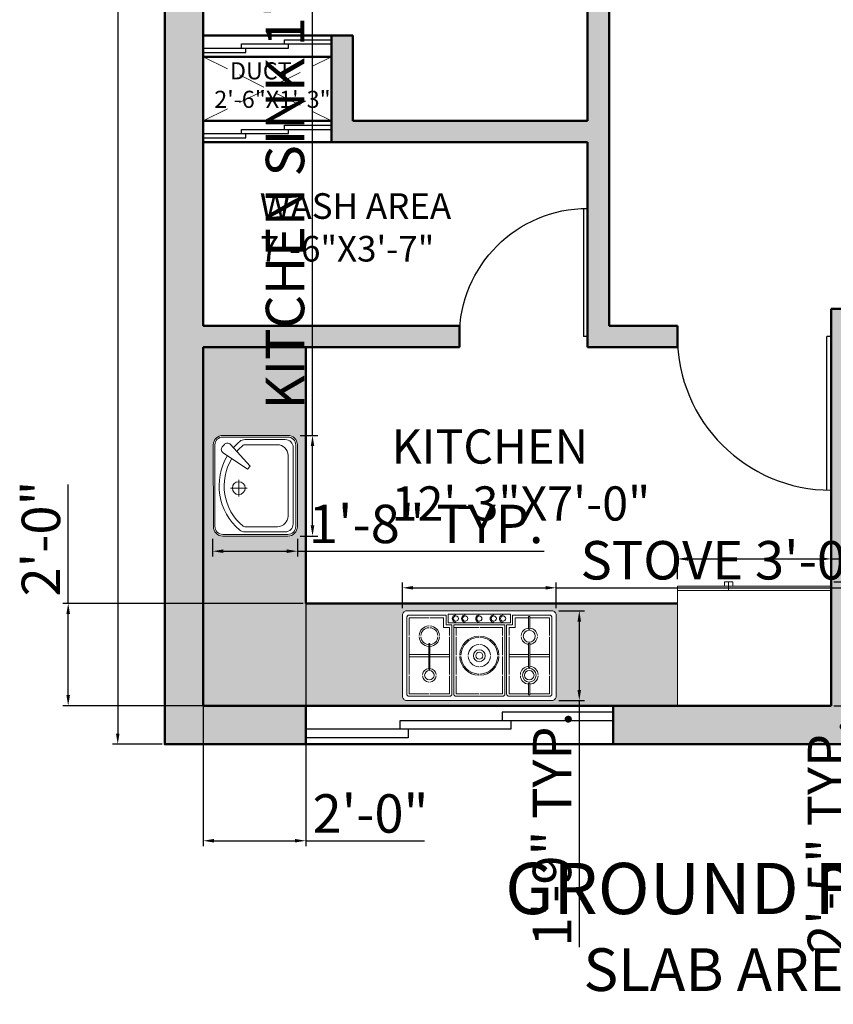
# Model space of a CAD drawing. Units: inches. Extents: x 3274 to 5176, y 1085 to 2172.
# Tile 5 of 16: x 3339 to 3530, y 1614 to 1844. Entities that reach past the tile are written whole.
import ezdxf

# ---------------------------------------------------------------- set-up
doc = ezdxf.new("R2010")
doc.units = ezdxf.units.IN
doc.linetypes.add('DASHED', pattern=[19.05, 12.7, -6.35])
for name, color, linetype, lineweight in [('A-ANNO-DIMS', 2, 'Continuous', 18), ('A-ANNO-TEXT', 7, 'Continuous', 25), ('A-AREA-IDEN', 3, 'Continuous', 25), ('A-DOOR', 4, 'Continuous', 25), ('A-FLOR-FIXT', 8, 'Continuous', 18), ('A-FLOR-OPEN', 7, 'DASHED', 18), ('A-FLOR-PATT', 252, 'Continuous', 13), ('A-GLAZ', 5, 'Continuous', 25), ('A-WALL', 7, 'Continuous', 50), ('A-WALL-PATT', 8, 'Continuous', 13)]:
    doc.layers.add(name, color=color, linetype=linetype, lineweight=lineweight)
doc.styles.get("Standard").update_dxf_attribs({"font": 'arial.ttf'})
doc.dimstyles.new('ISO-25', dxfattribs={"dimtxt": 9, "dimasz": 2.5, "dimexe": 1.25, "dimexo": 0.625, "dimtad": 1, "dimdec": 1, "dimlunit": 3, "dimtxsty": 'Standard', "dimcen": 2.5, "dimclrd": 4, "dimclre": 4, "dimclrt": 1, "dimadec": 0, "dimazin": 0, "dimtfac": 1, "dimtdec": 1, "dimtmove": 0, "dimatfit": 3, "dimfxl": 1, "dimarcsym": 0})

# ---------------------------------------------------------------- blocks, each defined once
blk = doc.blocks.new('2')
for p, q in [((0, 30), (0, 0)), ((1, 30), (1, 0)), ((0, 0), (1, 0))]:
    blk.add_line(p, q)
blk.add_arc((0, 0), 30, 0, 90)
blk = doc.blocks.new('1')
for p, q in [((0, 36), (0, 0)), ((1, 36), (1, 0)), ((0, 0), (1, 0))]:
    blk.add_line(p, q)
blk.add_arc((0, 0), 36, 0, 90)
blk = doc.blocks.new('*D68')
at = {"layer": 'A-ANNO-DIMS', "color": 0, "lineweight": -2, "transparency": 16777216}
for p, q in [((3372.68, 2034.48), (3361.05, 2034.48)), ((3362.3, 2031.98), (3362.3, 1676.98)), ((3372.68, 1674.48), (3361.05, 1674.48))]:
    blk.add_line(p, q, dxfattribs=at)
at = {"layer": 'A-ANNO-DIMS', "color": 0, "transparency": 16777216}
for points in [[(3361.88, 2031.98), (3362.71, 2031.98), (3362.3, 2034.48)], [(3361.88, 1676.98), (3362.71, 1676.98), (3362.3, 1674.48)]]:
    blk.add_solid(points, dxfattribs=at)
at = {"layer": 'Defpoints', "color": 0, "transparency": 16777216}
for p in [(3373.3, 2034.48), (3362.3, 1674.48), (3373.3, 1674.48)]:
    blk.add_point(p, dxfattribs=at)
at = {"layer": 'A-ANNO-DIMS', "color": 0, "transparency": 16777216, "insert": (3357.07, 1854.48), "char_height": 9, "attachment_point": 5, "rotation": 90}
blk.add_mtext("30'", dxfattribs=at)
blk = doc.blocks.new('STOVE')
for p, q in [((11.85, 19.7), (11.55, 19.7)), ((11.55, 16.92), (11.55, 19.7)), ((11.85, 16.92), (11.85, 19.7)), ((11.85, 16.92), (11.55, 16.92)), ((-11.85, 13.73), (-11.85, 7.62)), ((-11.85, 13.73), (-11.55, 13.73)), ((-11.55, 13.73), (-11.55, 7.62)), ((11.85, 13.23), (11.55, 13.23)), ((11.55, 13.23), (11.55, 7.57)), ((11.85, 13.23), (11.85, 7.57)), ((-11.85, 10.75), (-16.4, 10.75)), ((-11.85, 10.25), (-16.4, 10.25)), ((-7, 10.75), (-11.55, 10.75)), ((-7, 10.25), (-11.55, 10.25)), ((7, 10.75), (11.55, 10.75)), ((7, 10.25), (11.55, 10.25)), ((11.85, 10.75), (16.4, 10.75)), ((11.85, 10.25), (16.4, 10.25)), ((-11.85, 7.62), (-11.55, 7.62)), ((11.85, 7.57), (11.55, 7.57)), ((-7, 3.9), (-8.4, 3.9)), ((-7.8, 3.3), (-7.8, 1)), ((-6.4, 3.3), (-7.8, 3.3)), ((7.3, 2.8), (-7.3, 2.8)), ((-7.3, 2.8), (-7.3, 0.8)), ((-5.4, 3.9), (-6, 3.9)), ((-5.4, 3.9), (-0.15, 3.9)), ((0.15, 3.9), (5.4, 3.9)), ((6.4, 3.3), (7.8, 3.3)), ((7, 3.9), (8.4, 3.9)), ((7.3, 2.8), (7.3, 0.8)), ((7.8, 3.3), (7.8, 1)), ((8.4, 3.9), (8.4, 1.6)), ((11.85, 4.28), (11.55, 4.28)), ((11.55, 4.28), (11.55, 1.3)), ((11.85, 4.28), (11.85, 1.3)), ((7.3, 0.8), (-7.3, 0.8)), ((11.85, 1.3), (11.55, 1.3))]:
    blk.add_line(p, q)
for points in [[(-17, 21), (17, 21, -0.414214), (18, 20), (18, 1, -0.414214), (17, 0), (-17, 0, -0.414214), (-18, 1), (-18, 20, -0.414214)], [(6, 3.3), (-6, 3.3), (-6, 19.4, -0.414214), (-5.4, 20), (5.4, 20, -0.414214), (6, 19.4)]]:
    blk.add_lwpolyline(points, format="xyb", close=True)
for points in [[(-7.8, 1), (-16.4, 1, -0.414214), (-17, 1.6), (-17, 19.4, -0.414214), (-16.4, 20), (-7, 20, -0.414214), (-6.4, 19.4), (-6.4, 3.3)], [(6.4, 19.4, -0.414214), (7, 20), (16.4, 20, -0.414214), (17, 19.4), (17, 1.6, -0.414214), (16.4, 1), (7.8, 1)]]:
    blk.add_lwpolyline(points, format="xyb")
for points in [[(-16.4, 15.22), (-16.4, 19.4), (-11.85, 19.4)], [(-11.55, 19.4), (-7, 19.4), (-7, 15.22)], [(-5.4, 15.22), (-5.4, 19.4), (-0.15, 19.4)], [(0.15, 19.4), (5.4, 19.4), (5.4, 15.22)], [(6.4, 3.3), (6.4, 19.4)], [(7, 15.22), (7, 19.4), (11.55, 19.4)], [(11.85, 19.4), (16.4, 19.4), (16.4, 15.22)], [(-16.4, 6.08), (-16.4, 14.92)], [(-7, 14.92), (-7, 6.08)], [(-5.4, 10.65), (-5.4, 14.92)], [(5.4, 14.92), (5.4, 10.65)], [(7, 6.08), (7, 14.92)], [(16.4, 14.92), (16.4, 6.08)], [(-5.4, 6.08), (-5.4, 10.35)], [(5.4, 10.35), (5.4, 6.08)], [(-11.85, 1.6), (-16.4, 1.6), (-16.4, 5.77)], [(-7, 5.77), (-7, 3.9)], [(-5.4, 3.9), (-5.4, 5.77)], [(5.4, 5.77), (5.4, 3.9)], [(7, 3.9), (7, 5.77)], [(16.4, 5.77), (16.4, 1.6), (11.85, 1.6)], [(-8.4, 3.9), (-8.4, 1.6), (-11.55, 1.6)], [(11.55, 1.6), (8.4, 1.6)]]:
    blk.add_lwpolyline(points)
for centre, radius in [((-11.7, 15.07), 1.1), ((11.7, 15.07), 1.6), ((11.7, 15.07), 1.1), ((0, 10.5), 1.4), ((0, 10.5), 0.8), ((11.7, 5.93), 1.4), ((-5.49, 1.8), 0.6), ((-3.3, 1.8), 0.6), ((0, 1.8), 0.6), ((3.39, 1.8), 0.6), ((5.57, 1.8), 0.6)]:
    blk.add_circle(centre, radius)
for centre, radius, start, end in [((-11.7, 15.07), 1.6, 95.3794, 174.6206), ((-11.7, 15.07), 1.6, 5.3794, 84.6206), ((11.7, 15.07), 2.1, 94.096, 175.904), ((11.7, 15.07), 2.1, 4.096, 85.904), ((-11.7, 15.07), 1.6, 185.3794, 264.6206), ((-11.7, 15.07), 1.6, 275.3794, 354.6206), ((0, 10.5), 4.6, 91.8687, 178.1313), ((0, 10.5), 4.3, 91.9991, 178.0009), ((0, 10.5), 4.6, 1.8687, 88.1313), ((0, 10.5), 4.3, 1.9991, 88.0009), ((11.7, 15.07), 2.1, 184.096, 265.904), ((11.7, 15.07), 2.1, 274.096, 355.904), ((0, 10.5), 2.6, 93.3074, 176.6926), ((0, 10.5), 2.6, 3.3074, 86.6926), ((0, 10.5), 4.6, 181.8687, 268.1313), ((0, 10.5), 4.3, 181.9991, 268.0009), ((0, 10.5), 2.6, 183.3074, 266.6926), ((0, 10.5), 4.6, 271.8687, 358.1313), ((0, 10.5), 4.3, 271.9991, 358.0009), ((0, 10.5), 2.6, 273.3074, 356.6926), ((-11.7, 5.93), 2.4, 93.5833, 176.4167), ((-11.7, 5.93), 2, 94.3012, 175.6988), ((-11.7, 5.93), 2.4, 3.5833, 86.4167), ((-11.7, 5.93), 2, 4.3012, 85.6988), ((11.7, 5.93), 1.9, 94.5281, 175.4719), ((11.7, 5.93), 1.9, 4.5281, 85.4719), ((-11.7, 5.93), 2.4, 183.5833, 266.4167), ((-11.7, 5.93), 2, 184.3012, 265.6988), ((-11.7, 5.93), 2.4, 273.5833, 356.4167), ((-11.7, 5.93), 2, 274.3012, 355.6988), ((11.7, 5.93), 1.9, 184.5281, 265.4719), ((11.7, 5.93), 1.9, 274.5281, 355.4719), ((-5.49, 1.8), 0.846, 89.9979, 270), ((-3.3, 1.8), 0.846, 89.9979, 270), ((0, 1.8), 0.846, 89.9979, 270), ((3.39, 1.8), 0.846, 89.9979, 270), ((5.57, 1.8), 0.846, 89.9979, 270)]:
    blk.add_arc(centre, radius, start, end)
blk = doc.blocks.new('Refrigerator-2 door - 36 in top')
for p, q in [((0, -26.999999), (36, -26.999999)), ((12, -26.999999), (12, -28.999999)), ((11, -27.999999), (11, -28.999999)), ((11, -28.999999), (13, -28.999999)), ((13, -28.999999), (13, -27.999999))]:
    blk.add_line(p, q)
blk.add_lwpolyline([(0, -27.999999), (0, 0), (36, 0), (36, -27.999999)], close=True)
blk = doc.blocks.new('WIN-30')
for p, q in [((4375.19, 1317.35), (4396.19, 1317.35)), ((4375.19, 1316.35), (4375.19, 1317.35)), ((4385.19, 1318.35), (4396.19, 1318.35)), ((4385.19, 1317.35), (4385.19, 1318.35)), ((4386.19, 1316.35), (4386.19, 1317.35)), ((4366.19, 1316.35), (4386.19, 1316.35)), ((4366.19, 1315.35), (4376.19, 1315.35)), ((4376.19, 1315.35), (4376.19, 1316.35))]:
    blk.add_line(p, q)
blk = doc.blocks.new('WIN-72')
for p, q in [((4462.19, 1180.85), (4436.19, 1180.85)), ((4436.19, 1180.85), (4436.19, 1178.85)), ((4462.19, 1178.85), (4412.19, 1178.85)), ((4412.19, 1178.85), (4412.19, 1176.85)), ((4438.19, 1178.85), (4438.19, 1176.85)), ((4438.19, 1176.85), (4390.19, 1176.85)), ((4414.19, 1176.85), (4414.19, 1174.85)), ((4414.19, 1174.85), (4390.19, 1174.85))]:
    blk.add_line(p, q)
blk = doc.blocks.new('SINK-KITCHEN')
at = {"transparency": 33554687}
for points in [[(4388.24, 1243.45, 0.414214), (4386.01, 1245.69), (4370.78, 1245.67, 0.414214), (4368.55, 1243.47), (4368.57, 1224.32, 0.414214), (4370.77, 1222.1), (4386.01, 1222.1, 0.414214), (4388.24, 1224.33), (4388.24, 1243.45)], [(4387.87, 1243.45, 0.414214), (4386.01, 1245.3), (4370.78, 1245.3, 0.414214), (4368.94, 1243.47), (4368.94, 1224.32, 0.414214), (4370.77, 1222.5), (4386.01, 1222.5, 0.414214), (4387.84, 1224.33), (4387.87, 1243.45)], [(4371.89, 1240.94, 0.371519), (4374.75, 1223.51, 0.175764), (4375.92, 1223.1), (4385.42, 1223.08, 0.414214), (4387.24, 1224.93), (4387.27, 1242.85, 0.414214), (4385.41, 1244.69), (4375.92, 1244.69, 0.175764), (4374.75, 1244.27, 0.038632), (4373.27, 1242.81)], [(4372.88, 1240.28, 0.370401), (4375.51, 1224.41, 0.175764), (4375.92, 1224.28), (4383.57, 1224.28, 0.414214), (4386.06, 1226.79), (4386.06, 1241, 0.414214), (4383.55, 1243.51), (4375.92, 1243.51, 0.175764), (4375.51, 1243.36, 0.038512), (4374.06, 1241.92)]]:
    blk.add_lwpolyline(points, format="xyb", dxfattribs=at)
blk.add_lwpolyline([(4371.14, 1243.58), (4370.66, 1243, 0.463205), (4370.87, 1241.61), (4376.59, 1237.78), (4377.2, 1238.48), (4372.56, 1243.56, 0.4637)], format="xyb", close=True, dxfattribs=at)
for points in [[(4374.51, 1231.4), (4374.51, 1235.3)], [(4372.56, 1233.35), (4376.46, 1233.35)]]:
    blk.add_lwpolyline(points, dxfattribs=at)
blk.add_circle((4374.52, 1233.34), 1.5, dxfattribs=at)
blk = doc.blocks.new('*D134')
at = {"layer": 'A-ANNO-DIMS', "color": 4, "lineweight": -2, "transparency": 16777216}
for p, q in [((3428.94, 1706.35), (3428.94, 1712.37)), ((3431.44, 1711.12), (3462.44, 1711.12)), ((3464.94, 1706.35), (3464.94, 1712.37)), ((3464.94, 1711.12), (3569.61, 1711.12))]:
    blk.add_line(p, q, dxfattribs=at)
at = {"layer": 'A-ANNO-DIMS', "color": 4, "transparency": 16777216}
for points in [[(3431.44, 1711.54), (3431.44, 1710.7), (3428.94, 1711.12)], [(3462.44, 1711.54), (3462.44, 1710.7), (3464.94, 1711.12)]]:
    blk.add_solid(points, dxfattribs=at)
at = {"layer": 'Defpoints', "color": 0, "transparency": 16777216}
for p in [(3464.94, 1711.12), (3428.94, 1705.72), (3464.94, 1705.72)]:
    blk.add_point(p, dxfattribs=at)
at = {"layer": 'A-ANNO-DIMS', "color": 1, "transparency": 16777216, "insert": (3518.52, 1716.4), "char_height": 9, "attachment_point": 5}
blk.add_mtext('STOVE 3\'-0" TYP.', dxfattribs=at)
blk = doc.blocks.new('*D135')
at = {"layer": 'A-ANNO-DIMS', "color": 4, "lineweight": -2, "transparency": 16777216}
for p, q in [((3465.56, 1705.72), (3471.59, 1705.72)), ((3470.34, 1703.22), (3470.34, 1687.22)), ((3465.56, 1684.72), (3471.59, 1684.72)), ((3470.34, 1684.72), (3470.34, 1626.96))]:
    blk.add_line(p, q, dxfattribs=at)
at = {"layer": 'A-ANNO-DIMS', "color": 4, "transparency": 16777216}
for points in [[(3469.92, 1703.22), (3470.75, 1703.22), (3470.34, 1705.72)], [(3469.92, 1687.22), (3470.75, 1687.22), (3470.34, 1684.72)]]:
    blk.add_solid(points, dxfattribs=at)
at = {"layer": 'Defpoints', "color": 0, "transparency": 16777216}
for p in [(3464.94, 1705.72), (3464.94, 1684.72), (3470.34, 1684.72)]:
    blk.add_point(p, dxfattribs=at)
at = {"layer": 'A-ANNO-DIMS', "color": 1, "transparency": 16777216, "insert": (3465.12, 1654.59), "char_height": 9, "attachment_point": 5, "rotation": 90}
blk.add_mtext('1\'-9" TYP.', dxfattribs=at)
blk = doc.blocks.new('*D142')
at = {"layer": 'A-ANNO-DIMS', "color": 4, "lineweight": -2, "transparency": 16777216}
for p, q in [((3493.3, 1713.11), (3493.3, 1719.13)), ((3529.3, 1713.11), (3529.3, 1719.13)), ((3495.8, 1717.88), (3526.8, 1717.88)), ((3529.3, 1717.88), (3690.83, 1717.88))]:
    blk.add_line(p, q, dxfattribs=at)
at = {"layer": 'A-ANNO-DIMS', "color": 4, "transparency": 16777216}
for points in [[(3495.8, 1718.3), (3495.8, 1717.47), (3493.3, 1717.88)], [(3526.8, 1718.3), (3526.8, 1717.47), (3529.3, 1717.88)]]:
    blk.add_solid(points, dxfattribs=at)
at = {"layer": 'Defpoints', "color": 0, "transparency": 16777216}
for p in [(3529.3, 1717.88), (3493.3, 1712.48), (3529.3, 1712.48)]:
    blk.add_point(p, dxfattribs=at)
at = {"layer": 'A-ANNO-DIMS', "color": 1, "transparency": 16777216, "insert": (3611.31, 1723.17), "char_height": 9, "attachment_point": 5}
blk.add_mtext('REFRIGERATOR 3\'-0" TYP.', dxfattribs=at)
blk = doc.blocks.new('*D143')
at = {"layer": 'A-ANNO-DIMS', "color": 4, "lineweight": -2, "transparency": 16777216}
for p, q in [((3529.93, 1712.48), (3535.95, 1712.48)), ((3534.7, 1709.98), (3534.7, 1685.98)), ((3529.93, 1683.48), (3535.95, 1683.48)), ((3534.7, 1683.48), (3534.7, 1624.72))]:
    blk.add_line(p, q, dxfattribs=at)
at = {"layer": 'A-ANNO-DIMS', "color": 4, "transparency": 16777216}
for points in [[(3534.28, 1709.98), (3535.12, 1709.98), (3534.7, 1712.48)], [(3534.28, 1685.98), (3535.12, 1685.98), (3534.7, 1683.48)]]:
    blk.add_solid(points, dxfattribs=at)
at = {"layer": 'Defpoints', "color": 0, "transparency": 16777216}
for p in [(3529.3, 1712.48), (3529.3, 1683.48), (3534.7, 1683.48)]:
    blk.add_point(p, dxfattribs=at)
at = {"layer": 'A-ANNO-DIMS', "color": 1, "transparency": 16777216, "insert": (3529.48, 1652.85), "char_height": 9, "attachment_point": 5, "rotation": 90}
blk.add_mtext('2\'-5" TYP.', dxfattribs=at)
blk = doc.blocks.new('*D146')
at = {"layer": 'A-ANNO-DIMS', "color": 4, "lineweight": -2, "transparency": 16777216}
for p, q in [((3407.89, 1746.82), (3407.89, 1924.51)), ((3404.98, 1746.82), (3409.14, 1746.82)), ((3407.89, 1725.73), (3407.89, 1744.32)), ((3404.98, 1723.23), (3409.14, 1723.23))]:
    blk.add_line(p, q, dxfattribs=at)
at = {"layer": 'A-ANNO-DIMS', "color": 4, "transparency": 16777216}
for points in [[(3407.48, 1744.32), (3408.31, 1744.32), (3407.89, 1746.82)], [(3407.48, 1725.73), (3408.31, 1725.73), (3407.89, 1723.23)]]:
    blk.add_solid(points, dxfattribs=at)
at = {"layer": 'Defpoints', "color": 0, "transparency": 16777216}
for p in [(3404.36, 1746.82), (3407.89, 1746.82), (3404.36, 1723.23)]:
    blk.add_point(p, dxfattribs=at)
at = {"layer": 'A-ANNO-DIMS', "color": 1, "transparency": 16777216, "insert": (3402.62, 1836.92), "char_height": 9, "attachment_point": 5, "rotation": 90}
blk.add_mtext('KITCHEN SINK 1\'-11 1/2" TYP.', dxfattribs=at)
blk = doc.blocks.new('*D147')
at = {"layer": 'A-ANNO-DIMS', "color": 4, "lineweight": -2, "transparency": 16777216}
for p, q in [((3384.51, 1722.61), (3384.51, 1718.44)), ((3404.36, 1722.61), (3404.36, 1718.44)), ((3387.01, 1719.69), (3401.86, 1719.69)), ((3404.36, 1719.69), (3462.12, 1719.69))]:
    blk.add_line(p, q, dxfattribs=at)
at = {"layer": 'A-ANNO-DIMS', "color": 4, "transparency": 16777216}
for points in [[(3387.01, 1720.11), (3387.01, 1719.28), (3384.51, 1719.69)], [(3401.86, 1720.11), (3401.86, 1719.28), (3404.36, 1719.69)]]:
    blk.add_solid(points, dxfattribs=at)
at = {"layer": 'Defpoints', "color": 0, "transparency": 16777216}
for p in [(3384.51, 1723.23), (3404.36, 1723.23), (3404.36, 1719.69)]:
    blk.add_point(p, dxfattribs=at)
at = {"layer": 'A-ANNO-DIMS', "color": 1, "transparency": 16777216, "insert": (3434.49, 1724.91), "char_height": 9, "attachment_point": 5}
blk.add_mtext('1\'-8" TYP.', dxfattribs=at)
blk = doc.blocks.new('*D170')
at = {"layer": 'A-ANNO-DIMS', "color": 4, "lineweight": -2, "transparency": 16777216}
for p, q in [((3382.3, 1766.86), (3382.3, 1650.63)), ((3406.3, 1766.86), (3406.3, 1650.63)), ((3384.8, 1651.88), (3403.8, 1651.88)), ((3406.3, 1651.88), (3434.13, 1651.88))]:
    blk.add_line(p, q, dxfattribs=at)
at = {"layer": 'A-ANNO-DIMS', "color": 4, "transparency": 16777216}
for points in [[(3384.8, 1652.3), (3384.8, 1651.47), (3382.3, 1651.88)], [(3403.8, 1652.3), (3403.8, 1651.47), (3406.3, 1651.88)]]:
    blk.add_solid(points, dxfattribs=at)
at = {"layer": 'Defpoints', "color": 0, "transparency": 16777216}
for p in [(3382.3, 1767.48), (3406.3, 1767.48), (3406.3, 1651.88)]:
    blk.add_point(p, dxfattribs=at)
at = {"layer": 'A-ANNO-DIMS', "color": 1, "transparency": 16777216, "insert": (3421.46, 1657.1), "char_height": 9, "attachment_point": 5}
blk.add_mtext('2\'-0"', dxfattribs=at)
blk = doc.blocks.new('*D171')
at = {"layer": 'A-ANNO-DIMS', "color": 4, "lineweight": -2, "transparency": 16777216}
for p, q in [((3350.7, 1707.48), (3350.7, 1735.31)), ((3405.68, 1707.48), (3349.45, 1707.48)), ((3350.7, 1685.98), (3350.7, 1704.98)), ((3405.68, 1683.48), (3349.45, 1683.48))]:
    blk.add_line(p, q, dxfattribs=at)
at = {"layer": 'A-ANNO-DIMS', "color": 4, "transparency": 16777216}
for points in [[(3350.28, 1704.98), (3351.12, 1704.98), (3350.7, 1707.48)], [(3350.28, 1685.98), (3351.12, 1685.98), (3350.7, 1683.48)]]:
    blk.add_solid(points, dxfattribs=at)
at = {"layer": 'Defpoints', "color": 0, "transparency": 16777216}
for p in [(3350.7, 1707.48), (3406.3, 1707.48), (3406.3, 1683.48)]:
    blk.add_point(p, dxfattribs=at)
at = {"layer": 'A-ANNO-DIMS', "color": 1, "transparency": 16777216, "insert": (3345.48, 1722.65), "char_height": 9, "attachment_point": 5, "rotation": 90}
blk.add_mtext('2\'-0"', dxfattribs=at)

msp = doc.modelspace()

# ---------------------------------------------------------------- hatches: boundary and pattern name
at = {"layer": 'A-FLOR-PATT'}
h = msp.add_hatch(color=256, dxfattribs=at)
h.dxf.hatch_style = 1
h.paths.add_polyline_path([(3493.3, 1707.48), (3406.3, 1707.48), (3406.3, 1767.48), (3382.3, 1767.48), (3382.3, 1683.48), (3493.3, 1683.48)])
h.paths.add_polyline_path([(3404.35, 1725.46), (3404.35, 1744.59, 0.415106), (3402.11, 1746.82), (3386.86, 1746.8, 0.414031), (3384.66, 1744.55), (3384.68, 1725.43, 0.413504), (3386.9, 1723.23), (3402.13, 1723.23, 0.414214)], flags=16)
h.paths.add_polyline_path([(3386.89, 1723.63, -0.414214), (3385.05, 1725.45), (3385.05, 1744.58, -0.414214), (3386.89, 1746.43), (3402.13, 1746.43, -0.414214), (3403.98, 1744.58), (3403.96, 1725.46, -0.414214), (3402.13, 1723.63)], flags=0)
h.paths.add_polyline_path([(3392.04, 1724.23, -0.184883), (3390.82, 1724.68, -0.369938), (3388, 1742.06), (3386.98, 1742.74, -0.451108), (3386.75, 1744.1), (3387.23, 1744.68, -0.443262), (3388.6, 1744.76), (3389.37, 1743.92, -0.038991), (3390.86, 1745.39, -0.176171), (3392.04, 1745.82), (3401.52, 1745.82, -0.414214), (3403.38, 1743.98), (3403.36, 1726.06, -0.414214), (3401.53, 1724.21)], flags=0)
h.paths.add_polyline_path([(3389.14, 1734.48), (3390.62, 1734.48), (3390.62, 1735.97, 0.40968)], flags=0)
h.paths.add_polyline_path([(3428.94, 1704.72, -0.414214), (3429.94, 1705.72), (3463.94, 1705.72, -0.414214), (3464.94, 1704.72), (3464.94, 1685.72, -0.414214), (3463.94, 1684.72), (3429.94, 1684.72, -0.414214), (3428.94, 1685.72)], flags=16)
h.paths.add_polyline_path([(3429.94, 1704.12, -0.414214), (3430.54, 1704.72), (3439.14, 1704.72), (3439.14, 1702.42), (3440.54, 1702.42), (3440.54, 1686.32, -0.414214), (3439.94, 1685.72), (3430.54, 1685.72, -0.414214), (3429.94, 1686.32)], flags=0)
h.paths.add_polyline_path([(3429.94, 1699.95), (3430.54, 1699.95), (3430.54, 1704.12), (3435.09, 1704.12), (3435.09, 1704.42), (3435.39, 1704.42), (3438.54, 1704.12), (3438.54, 1701.82), (3439.94, 1701.82), (3439.94, 1699.95), (3440.54, 1699.95), (3440.54, 1699.65), (3439.94, 1699.65), (3439.94, 1690.8), (3440.54, 1690.8), (3440.54, 1690.5), (3439.94, 1690.5), (3439.94, 1686.32), (3435.39, 1686.32), (3435.39, 1686.02), (3435.09, 1686.02), (3430.54, 1686.32), (3430.54, 1690.5), (3429.94, 1690.5), (3429.94, 1690.8), (3430.54, 1690.8), (3430.54, 1699.65), (3429.94, 1699.65)], flags=0)
h.paths.add_polyline_path([(3435.39, 1702.19), (3435.39, 1701.79, -0.370891), (3437.23, 1699.95, -0.414214), (3435.39, 1697.8), (3435.39, 1697.4, 0.378035), (3437.63, 1699.65, 0.414214)], flags=0)
h.paths.add_polyline_path([(3435.09, 1689.05), (3435.09, 1689.56, -0.374693), (3434.14, 1690.65), (3433.66, 1690.36, 0.335495)], flags=0)
h.paths.add_polyline_path([(3439.64, 1702.92), (3439.64, 1704.92), (3454.24, 1704.92), (3454.24, 1702.92)], flags=0)
h.paths.add_polyline_path([(3442.05, 1703.92, -1), (3440.85, 1703.92, -1)], flags=0)
h.paths.add_polyline_path([(3440.94, 1702.42), (3452.94, 1702.42), (3452.94, 1686.32, -0.414214), (3452.34, 1685.72), (3441.54, 1685.72, -0.414214), (3440.94, 1686.32)], flags=0)
h.paths.add_polyline_path([(3440.94, 1699.95), (3441.54, 1699.95), (3441.54, 1701.82), (3446.79, 1701.82), (3446.79, 1702.12), (3447.09, 1702.12), (3452.34, 1701.82), (3452.34, 1699.95), (3452.94, 1699.95), (3452.94, 1699.65), (3452.34, 1699.65), (3452.34, 1695.37), (3452.64, 1695.37), (3452.64, 1695.07), (3452.34, 1690.8), (3452.94, 1690.8), (3452.94, 1690.5), (3452.34, 1690.5), (3452.34, 1686.32), (3447.09, 1686.32), (3447.09, 1686.02), (3446.79, 1686.02), (3441.54, 1686.32), (3441.54, 1690.5), (3440.94, 1690.5), (3440.94, 1690.8), (3441.54, 1690.8), (3441.54, 1695.07), (3441.24, 1695.07), (3441.24, 1695.37), (3441.54, 1699.65), (3440.94, 1699.65)], flags=0)
h.paths.add_polyline_path([(3447.09, 1699.82), (3447.09, 1699.52, -0.414214), (3451.23, 1695.07), (3451.53, 1695.07, 0.414214)], flags=0)
h.paths.add_polyline_path([(3444.34, 1695.37, -0.38079), (3446.79, 1697.82, -0.414214), (3449.53, 1695.37, -0.448446), (3446.79, 1692.62), (3446.79, 1690.62, -0.414214), (3442.34, 1695.37)], flags=0)
h.paths.add_polyline_path([(3444.24, 1703.92, -1), (3443.04, 1703.92, -1)], flags=0)
h.paths.add_polyline_path([(3448.34, 1695.22, -1), (3445.54, 1695.22, -1)], flags=0)
h.paths.add_polyline_path([(3447.54, 1703.92, -1), (3446.34, 1703.92, -1)], flags=0)
h.paths.add_polyline_path([(3447.74, 1695.22, -1), (3446.14, 1695.22, -1)], flags=0)
h.paths.add_polyline_path([(3450.92, 1703.92, -1), (3449.72, 1703.92, -1)], flags=0)
h.paths.add_polyline_path([(3453.11, 1703.92, -1), (3451.91, 1703.92, -1)], flags=0)
h.paths.add_polyline_path([(3453.34, 1702.42), (3454.74, 1702.42), (3454.74, 1704.72), (3463.34, 1704.72, -0.414214), (3463.94, 1704.12), (3463.94, 1686.32, -0.414214), (3463.34, 1685.72), (3453.94, 1685.72, -0.414214), (3453.34, 1686.32)], flags=0)
h.paths.add_polyline_path([(3453.34, 1699.95), (3453.94, 1699.95), (3453.94, 1701.82), (3455.34, 1701.82), (3455.34, 1704.12), (3458.49, 1704.12), (3458.49, 1704.42), (3458.79, 1704.42), (3463.34, 1704.12), (3463.34, 1699.95), (3463.94, 1699.95), (3463.94, 1699.65), (3463.34, 1699.65), (3463.34, 1690.8), (3463.94, 1690.8), (3463.94, 1690.5), (3463.34, 1690.5), (3463.34, 1686.32), (3458.79, 1686.32), (3458.79, 1686.02), (3458.49, 1686.02), (3453.94, 1686.32), (3453.94, 1690.5), (3453.34, 1690.5), (3453.34, 1690.8), (3453.94, 1690.8), (3453.94, 1699.65), (3453.34, 1699.65)], flags=0)
h.paths.add_polyline_path([(3458.79, 1701.69), (3458.79, 1701.19, -0.38311), (3460.04, 1699.8), (3460.51, 1700.09, 0.347071)], flags=0)
h.paths.add_polyline_path([(3458.49, 1688.55), (3458.49, 1689.05, -0.386974), (3457.04, 1690.65), (3456.56, 1690.35, 0.353316)], flags=0)
h.paths.add_polyline_path([(3458.49, 1698.15), (3458.79, 1698.15), (3458.79, 1692.49), (3458.49, 1692.49)], flags=0)
h.paths.add_polyline_path([(3459.74, 1690.65, -1), (3457.54, 1690.65, -1)], flags=0)
at = {"layer": 'A-WALL-PATT'}
h = msp.add_hatch(color=256, dxfattribs=at)
h.dxf.hatch_style = 1
h.paths.add_polyline_path([(3733.3, 2034.48), (3373.3, 2034.48), (3373.3, 1674.48), (3406.3, 1674.48), (3406.3, 1683.48), (3382.3, 1683.48), (3382.3, 1767.48), (3442.3, 1767.48), (3442.3, 1772.48), (3382.3, 1772.48), (3382.3, 1876.48), (3442.3, 1876.48), (3442.3, 1881.48), (3382.3, 1881.48), (3382.3, 2025.48), (3724.3, 2025.48), (3724.3, 1881.48), (3594.3, 1881.48), (3594.3, 1876.48), (3724.3, 1876.48), (3724.3, 1776.48), (3656.3, 1776.48), (3656.3, 1767.48), (3724.3, 1767.48), (3724.3, 1683.48), (3682.3, 1683.48), (3682.3, 1674.48), (3733.3, 1674.48)])
h.paths.add_polyline_path([(3477.3, 1876.48), (3493.3, 1876.48), (3493.3, 1881.48), (3472.3, 1881.48), (3472.3, 1820.48), (3417.3, 1820.48), (3417.3, 1840.48), (3412.3, 1840.48), (3412.3, 1815.48), (3472.3, 1815.48), (3472.3, 1767.48), (3493.3, 1767.48), (3493.3, 1772.48), (3477.3, 1772.48)], flags=17)
h.paths.add_polyline_path([(3534.3, 1984.48), (3552.3, 1984.48), (3552.3, 1989.48), (3529.3, 1989.48), (3529.3, 1876.48), (3552.3, 1876.48), (3552.3, 1881.48), (3534.3, 1881.48), (3534.3, 1919.48), (3564.3, 1919.48), (3564.3, 1924.48), (3534.3, 1924.48)], flags=17)
h.paths.add_polyline_path([(3599.3, 1989.48), (3576.3, 1989.48), (3576.3, 1984.48), (3594.3, 1984.48), (3594.3, 1917.48), (3599.3, 1917.48)], flags=17)
h.paths.add_polyline_path([(3534.3, 1767.48), (3539.3, 1767.48), (3539.3, 1776.48), (3529.3, 1776.48), (3529.3, 1683.48), (3478.3, 1683.48), (3478.3, 1674.48), (3534.3, 1674.48)], flags=17)
h.paths.add_polyline_path([(3596.3, 1776.48), (3587.3, 1776.48), (3587.3, 1771.98), (3587.3, 1767.48), (3596.3, 1767.48)], flags=17)
h.paths.add_polyline_path([(3610.3, 1683.48), (3594.3, 1683.48), (3594.3, 1674.48), (3610.3, 1674.48)], flags=17)
h.paths.add_polyline_path([(3589.35, 1817.42), (3663.55, 1817.42), (3663.55, 1847.27), (3589.35, 1847.27)], flags=25)
h.paths.add_polyline_path([(3545.54, 1954.13), (3584.72, 1954.13), (3584.72, 1976.52), (3545.54, 1976.52)], flags=25)
h.paths.add_polyline_path([(3635.11, 1944.89), (3703.51, 1944.89), (3703.51, 1974.74), (3635.11, 1974.74)], flags=25)
h.paths.add_polyline_path([(3543.78, 1998.17), (3585.75, 1998.17), (3585.75, 2020.56), (3543.78, 2020.56)], flags=25)
h.paths.add_polyline_path([(3423.19, 1944.89), (3491.58, 1944.89), (3491.58, 1974.74), (3423.19, 1974.74)], flags=25)

# ---------------------------------------------------------------- linework, layer by layer
at = {"layer": 'A-FLOR-OPEN', "ltscale": 0.5}
for p, q in [((3382.3, 1835.48), (3412.3, 1820.48)), ((3382.3, 1820.48), (3412.3, 1835.48))]:
    msp.add_line(p, q, dxfattribs=at)
at = {"layer": 'A-WALL'}
for p, q in [((3472.3, 1820.48), (3472.3, 1881.48)), ((3382.3, 1772.48), (3382.3, 1876.48)), ((3477.3, 1772.48), (3477.3, 1876.48)), ((3382.3, 1840.48), (3417.3, 1840.48)), ((3412.3, 1815.48), (3412.3, 1840.48)), ((3417.3, 1820.48), (3417.3, 1840.48)), ((3382.3, 1835.48), (3412.3, 1835.48)), ((3382.3, 1820.48), (3412.3, 1820.48)), ((3417.3, 1820.48), (3472.3, 1820.48)), ((3382.3, 1815.48), (3472.3, 1815.48)), ((3472.3, 1767.48), (3472.3, 1815.48)), ((3529.3, 1776.48), (3539.3, 1776.48)), ((3529.3, 1683.48), (3529.3, 1776.48)), ((3382.3, 1772.48), (3442.3, 1772.48)), ((3442.3, 1767.48), (3442.3, 1772.48)), ((3477.3, 1772.48), (3493.3, 1772.48)), ((3493.3, 1767.48), (3493.3, 1772.48)), ((3382.3, 1767.48), (3442.3, 1767.48)), ((3382.3, 1683.48), (3382.3, 1767.48)), ((3406.3, 1707.48), (3406.3, 1767.48)), ((3472.3, 1767.48), (3493.3, 1767.48)), ((3493.3, 1707.48), (3406.3, 1707.48)), ((3529.3, 1683.48), (3382.3, 1683.48)), ((3406.3, 1683.48), (3406.3, 1674.48)), ((3478.3, 1683.48), (3478.3, 1674.48))]:
    msp.add_line(p, q, dxfattribs=at)
msp.add_lwpolyline([(3534.3, 1674.48), (3373.3, 1674.48), (3373.3, 2034.48), (3733.3, 2034.48), (3733.3, 1674.48), (3594.3, 1674.48)], dxfattribs=at)

# ---------------------------------------------------------------- block references
at = {"layer": 'A-DOOR', "xscale": -1}
msp.add_blockref('2', (3472.3, 1769.98), dxfattribs=at)
at = {"layer": 'A-DOOR', "rotation": 180}
msp.add_blockref('1', (3529.3, 1769.98), dxfattribs=at)
at = {"layer": 'A-FLOR-FIXT'}
msp.add_blockref('SINK-KITCHEN', (-983.89, 501.13), dxfattribs=at)
at = {"layer": 'A-FLOR-FIXT', "xscale": -1, "rotation": 180}
for name, p in [('Refrigerator-2 door - 36 in top', (3493.3, 1683.48)), ('STOVE', (3446.94, 1705.72))]:
    msp.add_blockref(name, p, dxfattribs=at)
at = {"layer": 'A-GLAZ'}
for name, p in [('WIN-30', (-983.89, 521.13)), ('WIN-30', (-983.89, 501.13)), ('WIN-72', (-983.89, 501.13))]:
    msp.add_blockref(name, p, dxfattribs=at)

# ---------------------------------------------------------------- texts
at = {"layer": 'A-ANNO-TEXT', "insert": (3452.99, 1646.7), "char_height": 12, "attachment_point": 1}
msp.add_mtext_dynamic_manual_height_columns('GROUND FLOOR PLAN\\P{\\H0.83333x;      SLAB AREA-900Sq.ft}', width=202.3193, gutter_width=30, heights=[0], dxfattribs=at)
at = {"layer": 'A-AREA-IDEN', "attachment_point": 1}
for s, heights, insert, char_height in [('   DUCT\\P2\'-6"X1\'-3"', [16.24], (3384.9, 1834.19), 4), ('WASH AREA\\P7\'-6"X3\'-7"', [0], (3395.55, 1803.53), 6), ('KITCHEN\\P12\'-3"X7\'-0"', [0], (3426.41, 1748.21), 8)]:
    msp.add_mtext_dynamic_manual_height_columns(s, width=58.0121, gutter_width=30, heights=heights, dxfattribs=dict(at, insert=insert, char_height=char_height))

# ---------------------------------------------------------------- dimensions: what is measured, and where the dimension line sits
at = {"layer": 'A-ANNO-DIMS'}
for base, p1, p2, override, picture, middle in [((3362.3, 1674.48), (3373.3, 2034.48), (3373.3, 1674.48), {"dimclrd": 0, "dimclre": 0, "dimclrt": 0}, '*D68', (3357.07, 1854.48)), ((3350.7, 1707.48), (3406.3, 1683.48), (3406.3, 1707.48), {"dimdec": 1, "dimlfac": 1, "dimrnd": 0, "dimzin": 1, "dimdsep": 46, "dimlunit": 4, "dimfrac": 2}, '*D171', (3345.48, 1722.65))]:
    dim = msp.add_linear_dim(base=base, p1=p1, p2=p2, angle=90, dimstyle='ISO-25', override=override, dxfattribs=at)
    dim.commit()
    dim.dimension.update_dxf_attribs({"geometry": picture, "text_midpoint": middle})
for base, p1, p2, angle, text, picture, middle in [((3407.89, 1746.82), (3404.36, 1723.23), (3404.36, 1746.82), 90, 'KITCHEN SINK <> TYP.', '*D146', (3402.62, 1836.92)), ((3534.7, 1683.48), (3529.3, 1712.48), (3529.3, 1683.48), 270, '<> TYP.', '*D143', (3529.48, 1652.85)), ((3470.34, 1684.72), (3464.94, 1705.72), (3464.94, 1684.72), 270, '<> TYP.', '*D135', (3465.12, 1654.59))]:
    dim = msp.add_linear_dim(base=base, p1=p1, p2=p2, angle=angle, text=text, dimstyle='ISO-25', override={"dimdec": 1, "dimrnd": 0, "dimzin": 1, "dimlunit": 4, "dimfrac": 2}, dxfattribs=at)
    dim.commit()
    dim.dimension.update_dxf_attribs({"geometry": picture, "text_midpoint": middle})
dim = msp.add_linear_dim(base=(3406.3, 1651.88), p1=(3382.3, 1767.48), p2=(3406.3, 1767.48), dimstyle='ISO-25', override={"dimdec": 1, "dimlfac": 1, "dimrnd": 0, "dimzin": 1, "dimdsep": 46, "dimlunit": 4, "dimfrac": 2}, dxfattribs=at)
dim.commit()
dim.dimension.update_dxf_attribs({"geometry": '*D170', "text_midpoint": (3421.46, 1657.1)})
for base, p1, p2, text, picture, middle in [((3529.3, 1717.88), (3493.3, 1712.48), (3529.3, 1712.48), 'REFRIGERATOR <> TYP.', '*D142', (3611.31, 1723.17)), ((3404.3562, 1719.6929), (3384.5107, 1723.2314), (3404.3562, 1723.2314), '<> TYP.', '*D147', (3434.4874, 1724.913)), ((3464.94, 1711.12), (3428.94, 1705.72), (3464.94, 1705.72), 'STOVE <> TYP.', '*D134', (3518.52, 1716.4))]:
    dim = msp.add_linear_dim(base=base, p1=p1, p2=p2, text=text, dimstyle='ISO-25', override={"dimdec": 1, "dimrnd": 0, "dimzin": 1, "dimlunit": 4, "dimfrac": 2}, dxfattribs=at)
    dim.commit()
    dim.dimension.update_dxf_attribs({"geometry": picture, "text_midpoint": middle})

doc.saveas('drawing.dxf')
